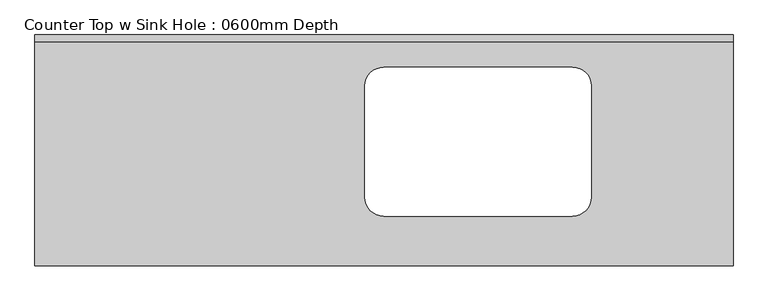
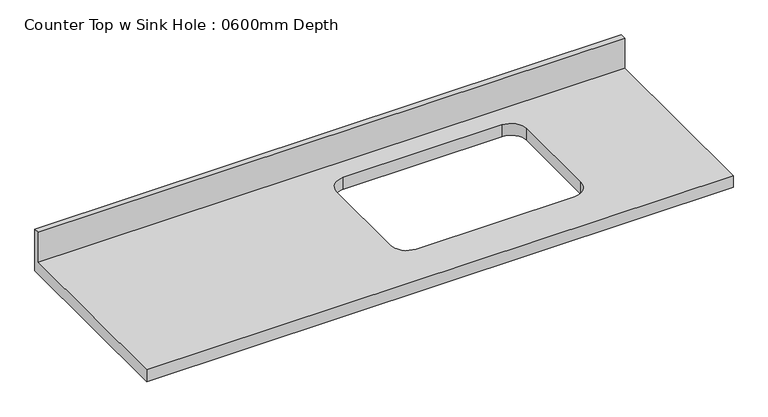
"""IFC4 building model written with IfcOpenShell, lengths in millimetres: furniture geometry, Counter Top w Sink Hole : 0600mm Depth."""

from ifc_helpers import new_model, si_unit, frame, origin, place, context, project, spatial, polyline, circle_curve, source, transform, mapped, element, save
from ifc_brep_helpers import plane_surface, revolved_surface, advanced_brep


def counter_top_w_sink_hole_0600mm_depth_1dfd4d8d(model_context):
    return source(origin(), model_context, "Body", "AdvancedBrep", [
        advanced_brep(
        [(-1200.4622951, -624.68125, 900.1125), (690.2502049, -624.68125, 900.1125), (690.2502049, -19.05, 900.1125), (-1200.4622951, -19.05, 900.1125), (-255.8997951, -87.3125, 900.1125), (255.2752049, -87.3125, 900.1125), (306.0752049, -138.1125, 900.1125), (306.0752049, -439.7375, 900.1125), (255.2752049, -490.5375, 900.1125), (-255.8997951, -490.5375, 900.1125), (-306.6997951, -439.7375, 900.1125), (-306.6997951, -138.1125, 900.1125), (690.2502049, 0.0, 860.425), (690.2502049, -624.68125, 860.425), (-1200.4622951, -624.68125, 860.425), (-1200.4622951, 0.0, 860.425), (255.2752049, -87.3125, 860.425), (-255.8997951, -87.3125, 860.425), (-306.6997951, -138.1125, 860.425), (-306.6997951, -439.7375, 860.425), (-255.8997951, -490.5375, 860.425), (255.2752049, -490.5375, 860.425), (306.0752049, -439.7375, 860.425), (306.0752049, -138.1125, 860.425), (-1200.4622951, 0.0, 1001.7125), (690.2502049, 0.0, 1001.7125), (-1200.4622951, -19.05, 1001.7125), (690.2502049, -19.05, 1001.7125)],
        [
            (0, 1),
            (1, 2),
            (2, 3),
            (3, 0),
            (4, 5),
            (5, 6, circle_curve(frame((255.2752049, -138.1125, 900.1125), z_axis=(0.0, 0.0, -1.0), x_axis=(1.0, 0.0, 0.0)), 50.8)),
            (6, 7),
            (7, 8, circle_curve(frame((255.2752049, -439.7375, 900.1125), z_axis=(0.0, 0.0, -1.0), x_axis=(1.0, 0.0, 0.0)), 50.8)),
            (8, 9),
            (9, 10, circle_curve(frame((-255.8997951, -439.7375, 900.1125), z_axis=(0.0, 0.0, -1.0), x_axis=(1.0, 0.0, 0.0)), 50.8)),
            (10, 11),
            (11, 4, circle_curve(frame((-255.8997951, -138.1125, 900.1125), z_axis=(0.0, 0.0, -1.0), x_axis=(1.0, 0.0, 0.0)), 50.8)),
            (12, 13),
            (13, 14),
            (14, 15),
            (15, 12),
            (16, 17),
            (17, 18, circle_curve(frame((-255.8997951, -138.1125, 860.425), z_axis=(0.0, 0.0, 1.0), x_axis=(1.0, 0.0, 0.0)), 50.8)),
            (18, 19),
            (19, 20, circle_curve(frame((-255.8997951, -439.7375, 860.425), z_axis=(0.0, 0.0, 1.0), x_axis=(1.0, 0.0, 0.0)), 50.8)),
            (20, 21),
            (21, 22, circle_curve(frame((255.2752049, -439.7375, 860.425), z_axis=(0.0, 0.0, 1.0), x_axis=(1.0, 0.0, 0.0)), 50.8)),
            (22, 23),
            (23, 16, circle_curve(frame((255.2752049, -138.1125, 860.425), z_axis=(0.0, 0.0, 1.0), x_axis=(1.0, 0.0, 0.0)), 50.8)),
            (15, 24),
            (24, 25),
            (25, 12),
            (14, 0),
            (3, 26),
            (26, 24),
            (13, 1),
            (25, 27),
            (27, 2),
            (4, 17),
            (16, 5),
            (11, 18),
            (10, 19),
            (9, 20),
            (8, 21),
            (7, 22),
            (6, 23),
            (26, 27),
        ],
        [
            plane_surface(frame((-1200.4622951, 0.0, 900.1125), z_axis=(0.0, 0.0, 1.0), x_axis=(-1.0, 0.0, 0.0))),
            plane_surface(frame((-1200.4622951, 0.0, 860.425), z_axis=(0.0, 0.0, -1.0), x_axis=(1.0, 0.0, 0.0))),
            plane_surface(frame((690.2502049, 0.0, 900.1125), z_axis=(0.0, 1.0, 0.0), x_axis=(0.0, 0.0, -1.0))),
            plane_surface(frame((-1200.4622951, 0.0, 900.1125), z_axis=(-1.0, 0.0, 0.0), x_axis=(0.0, 0.0, -1.0))),
            plane_surface(frame((-1200.4622951, -624.68125, 900.1125), z_axis=(0.0, -1.0, 0.0), x_axis=(0.0, 0.0, -1.0))),
            plane_surface(frame((690.2502049, -624.68125, 900.1125), z_axis=(1.0, 0.0, 0.0), x_axis=(0.0, 0.0, -1.0))),
            plane_surface(frame((255.2752049, -87.3125, 900.1125), z_axis=(0.0, -1.0, 0.0), x_axis=(0.0, 0.0, -1.0))),
            revolved_surface(polyline([(-205.0997951, -138.1125, 900.1125), (-205.0997951, -138.1125, 860.425)]), (-255.8997951, -138.1125, 860.425), (0.0, 0.0, 1.0)),
            plane_surface(frame((-306.6997951, -138.1125, 900.1125), z_axis=(1.0, 0.0, 0.0), x_axis=(0.0, 0.0, -1.0))),
            revolved_surface(polyline([(-205.0997951, -439.7375, 900.1125), (-205.0997951, -439.7375, 860.425)]), (-255.8997951, -439.7375, 860.425), (0.0, 0.0, 1.0)),
            plane_surface(frame((-255.8997951, -490.5375, 900.1125), z_axis=(0.0, 1.0, 0.0), x_axis=(0.0, 0.0, -1.0))),
            revolved_surface(polyline([(306.0752049, -439.7375, 900.1125), (306.0752049, -439.7375, 860.425)]), (255.2752049, -439.7375, 860.425), (0.0, 0.0, 1.0)),
            plane_surface(frame((306.0752049, -439.7375, 900.1125), z_axis=(-1.0, 0.0, 0.0), x_axis=(0.0, 0.0, -1.0))),
            revolved_surface(polyline([(306.0752049, -138.1125, 900.1125), (306.0752049, -138.1125, 860.425)]), (255.2752049, -138.1125, 860.425), (0.0, 0.0, 1.0)),
            plane_surface(frame((-1200.4622951, 0.0, 1001.7125), z_axis=(0.0, 0.0, 1.0), x_axis=(0.0, -1.0, 0.0))),
            plane_surface(frame((-1200.4622951, -19.05, 1001.7125), z_axis=(0.0, -1.0, 0.0), x_axis=(0.0, 0.0, -1.0))),
        ],
        [
            (0, [[1, 2, 3, 4], [5, 6, 7, 8, 9, 10, 11, 12]]),
            (1, [[13, 14, 15, 16], [17, 18, 19, 20, 21, 22, 23, 24]]),
            (2, [[-16, 25, 26, 27]]),
            (3, [[-15, 28, -4, 29, 30, -25]]),
            (4, [[-1, -28, -14, 31]]),
            (5, [[-13, -27, 32, 33, -2, -31]]),
            (6, [[34, -17, 35, -5]]),
            (7, [[-34, -12, 36, -18]]),
            (8, [[-36, -11, 37, -19]]),
            (9, [[-37, -10, 38, -20]]),
            (10, [[-38, -9, 39, -21]]),
            (11, [[-39, -8, 40, -22]]),
            (12, [[-40, -7, 41, -23]]),
            (13, [[-35, -24, -41, -6]]),
            (14, [[-30, 42, -32, -26]]),
            (15, [[-42, -29, -3, -33]]),
        ],
    ),
    ])


if __name__ == "__main__":
    model = new_model("IFC4")
    model_context = context("Model", 3, world=origin())
    ifc_project = project(units=[si_unit("LENGTHUNIT", "METRE", prefix="MILLI")], contexts=[model_context])
    site = spatial("IfcSite", under=ifc_project)
    building = spatial("IfcBuilding", under=site)
    placement = place(None, origin())
    counter_top_w_sink_hole_0600mm_depth_shape = counter_top_w_sink_hole_0600mm_depth_1dfd4d8d(model_context)
    element("IfcFurniture", 1, ObjectType="Counter Top w Sink Hole : 0600mm Depth", at=placement, inside=building, context=model_context, shape_type="MappedRepresentation", body=[
        mapped(counter_top_w_sink_hole_0600mm_depth_shape, transform((0.0, 0.0, 0.0), x_axis=(1.0, 0.0, 0.0), y_axis=(0.0, 1.0, 0.0), z_axis=(0.0, 0.0, 1.0))),
    ])
    save(model, "model.ifc")

# Revit data of these elements
# Type "Counter Top w Sink Hole : 0600mm Depth"
#   Assembly Code = "C1030400"
#   Counter Thickness = 0' - 1 9/16"
#   Depth = 2' - 0 19/32"
#   Height = 2' - 11 7/16"
#   Length [instance default] = 8' - 2 7/16"
#   Sink Location [instance default] = 3' - 11 1/4"
#   Sink Location To Wall [instance default] = 0' - 3 15/16"
#   Sink Opening Depth [instance default] = 1' - 2 7/8"
#   Sink Opening Width [instance default] = 1' - 11 1/8"
#   Counter Top Material = none
#   Default Elevation = 0
# Element 1 (IfcFurniture, "Counter Top w Sink Hole : 0600mm Depth")
#   Length = 6' - 2 7/16"
#   Materials on its faces: "Counter Top"
# Materials
#   "Counter Top": class "Wood", colour RGB 226 177 128, transparency 0
